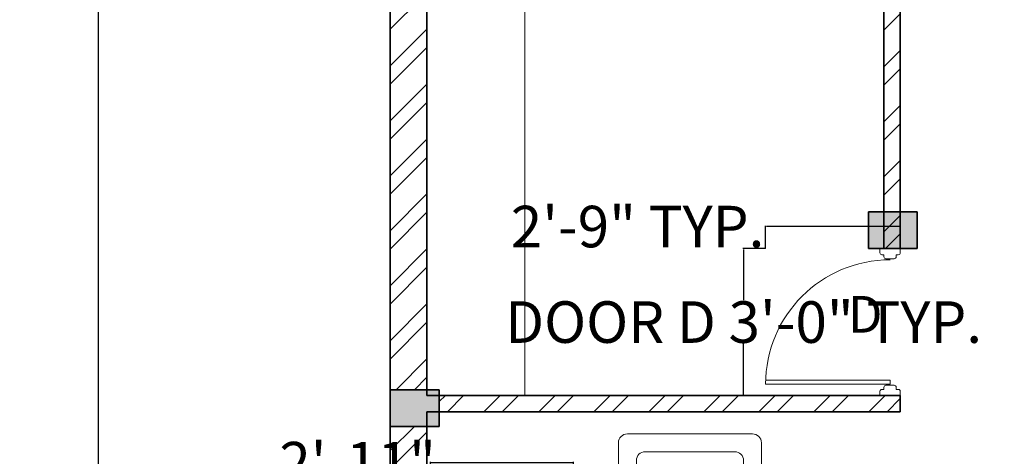
# Model space of a CAD drawing. Units: inches. Extents: x 2379 to 3013, y 1431 to 2110.
# Tile 3 of 10: x 2379 to 2620, y 1795 to 1902. Entities that reach past the tile are written whole.
import ezdxf

# ---------------------------------------------------------------- set-up
doc = ezdxf.new("R2010")
doc.units = ezdxf.units.IN
for name, color, linetype, lineweight in [('00 FURNITURE', 15, 'Continuous', 15), ('A-ANNO-DIMS', 2, 'Continuous', 18), ('A-ANNO-TEXT', 7, 'Continuous', 18), ('A-COLS', 7, 'Continuous', 35), ('A-COLS-PATT', 252, 'Continuous', 13), ('A-DOOR', 4, 'Continuous', 18), ('A-FLOR-CASE', 8, 'Continuous', 18), ('A-WALL-PATT', 8, 'Continuous', 13), ('WALL', 7, 'Continuous', 35)]:
    doc.layers.add(name, color=color, linetype=linetype, lineweight=lineweight)
doc.styles.get("Standard").update_dxf_attribs({"font": 'arial.ttf'})
doc.dimstyles.get("Standard").update_dxf_attribs({"dimtxt": 10.18, "dimasz": 0.18, "dimexe": 0.18, "dimexo": 0.0625, "dimgap": 0.09, "dimtad": 0, "dimtih": 1, "dimtoh": 1, "dimdec": 0, "dimzin": 0, "dimdsep": 46, "dimlunit": 3, "dimtxsty": 'Standard', "dimcen": 0.09, "dimadec": 0, "dimazin": 0, "dimtfac": 1, "dimtdec": 0, "dimtofl": 0, "dimtmove": 0, "dimatfit": 3, "dimfxl": 1, "dimtolj": 1, "dimtzin": 0, "dimarcsym": 0})

# ---------------------------------------------------------------- blocks, each defined once
blk = doc.blocks.new('column')
for p, q in [((2588.21, 2021.79), (2597.21, 2021.79)), ((2588.21, 2009.79), (2588.21, 2021.79)), ((2597.21, 2021.79), (2597.21, 2009.79)), ((2597.21, 2009.79), (2588.21, 2009.79))]:
    blk.add_line(p, q)
blk = doc.blocks.new('DDD')
at = {"layer": '00 FURNITURE'}
for p, q in [((-12579.77, -15859.53), (-12579.77, -15829.05)), ((-12578.77, -15859.53), (-12578.77, -15829.03)), ((-12612.02, -15857.03), (-12612.02, -15862.03)), ((-12611.02, -15857.03), (-12612.02, -15857.03)), ((-12577.02, -15857.03), (-12576.02, -15857.03)), ((-12576.02, -15857.03), (-12576.02, -15862.03)), ((-12610.52, -15858.03), (-12610.52, -15857.53)), ((-12578.77, -15859.53), (-12579.77, -15859.53)), ((-12577.52, -15858.03), (-12577.52, -15857.53)), ((-12612.02, -15862.03), (-12611.02, -15862.03)), ((-12610.52, -15861.53), (-12610.52, -15861.03)), ((-12577.52, -15861.53), (-12577.52, -15861.03)), ((-12576.02, -15862.03), (-12577.02, -15862.03))]:
    blk.add_line(p, q, dxfattribs=at)
for points in [[(-12610.52, -15861.03), (-12610.02, -15861.03, 0.414214), (-12609.52, -15860.53), (-12609.52, -15858.53, 0.414214), (-12610.02, -15858.03), (-12610.52, -15858.03)], [(-12577.52, -15861.03), (-12578.02, -15861.03, -0.414214), (-12578.52, -15860.53), (-12578.52, -15858.53, -0.414214), (-12578.02, -15858.03), (-12577.52, -15858.03)]]:
    blk.add_lwpolyline(points, format="xyb", dxfattribs=at)
for centre, radius, start, end in [((-12578.77, -15859.53), 30.5, 90, 180), ((-12611.02, -15857.53), 0.5, 0, 90), ((-12577.02, -15857.53), 0.5, 90, 180), ((-12611.02, -15861.53), 0.5, 270, 0), ((-12577.02, -15861.53), 0.5, 180, 270)]:
    blk.add_arc(centre, radius, start, end, dxfattribs=at)
blk = doc.blocks.new('*D13')
at = {"layer": 'A-ANNO-DIMS', "color": 0, "lineweight": -2, "transparency": 16777216}
for p, q in [((2469.57, 2021.61), (2397.82, 2021.61)), ((2398, 2021.43), (2398, 1755.4)), ((2398, 1478.79), (2398, 1744.82)), ((2469.57, 1478.61), (2397.82, 1478.61))]:
    blk.add_line(p, q, dxfattribs=at)
at = {"layer": 'A-ANNO-DIMS', "color": 0, "transparency": 16777216}
for points in [[(2397.97, 2021.43), (2398.03, 2021.43), (2398, 2021.61)], [(2397.97, 1478.79), (2398.03, 1478.79), (2398, 1478.61)]]:
    blk.add_solid(points, dxfattribs=at)
at = {"layer": 'Defpoints', "color": 0, "transparency": 16777216}
for p in [(2469.63, 2021.61), (2398, 1478.61), (2469.63, 1478.61)]:
    blk.add_point(p, dxfattribs=at)
at = {"layer": 'A-ANNO-DIMS', "color": 0, "transparency": 16777216, "insert": (2398, 1750.11), "char_height": 10.18, "attachment_point": 5}
blk.add_mtext('\\A1;45\'-3"', dxfattribs=at)
blk = doc.blocks.new('CHAIR-LOUNGE')
for p, q in [((32.85, 35.04), (2.19, 35.04)), ((0, 32.85), (0, 6.57)), ((35.04, 6.57), (35.04, 32.85)), ((28.47, 30.66), (6.57, 30.66)), ((4.38, 28.47), (4.38, 2.19)), ((30.66, 2.19), (30.66, 28.47)), ((30.66, 26.28), (4.38, 26.28)), ((2.19, 4.38), (4.38, 4.38)), ((30.66, 4.38), (32.85, 4.38)), ((6.57, 0), (28.47, 0))]:
    blk.add_line(p, q)
for centre, start, end in [((2.19, 32.85), 90, 180), ((32.85, 32.85), 0, 90), ((6.57, 28.47), 90, 180), ((28.47, 28.47), 0, 90), ((2.19, 6.57), 180, 270), ((32.85, 6.57), 270, 0), ((6.57, 2.19), 180, 270), ((28.47, 2.19), 270, 0)]:
    blk.add_arc(centre, 2.19, start, end)
blk = doc.blocks.new('*D24')
at = {"layer": 'A-ANNO-DIMS', "color": 0, "lineweight": -2, "transparency": 16777216}
for p, q in [((2561.57, 1845.61), (2556.05, 1845.61)), ((2556.23, 1845.43), (2556.23, 1832.97)), ((2556.23, 1809.79), (2556.23, 1822.25)), ((2561.57, 1809.61), (2556.05, 1809.61))]:
    blk.add_line(p, q, dxfattribs=at)
at = {"layer": 'A-ANNO-DIMS', "color": 0, "transparency": 16777216}
for points in [[(2556.2, 1845.43), (2556.26, 1845.43), (2556.23, 1845.61)], [(2556.2, 1809.79), (2556.26, 1809.79), (2556.23, 1809.61)]]:
    blk.add_solid(points, dxfattribs=at)
at = {"layer": 'Defpoints', "color": 0, "transparency": 16777216}
for p in [(2561.63, 1845.61), (2556.23, 1809.61), (2561.63, 1809.61)]:
    blk.add_point(p, dxfattribs=at)
at = {"layer": 'A-ANNO-DIMS', "color": 0, "transparency": 16777216, "insert": (2556.23, 1827.61), "char_height": 10.18, "attachment_point": 5}
blk.add_mtext('\\A1;DOOR D 3\'-0" TYP.', dxfattribs=at)
blk = doc.blocks.new('*D25')
at = {"layer": 'A-ANNO-DIMS', "color": 0, "lineweight": -2, "transparency": 16777216}
for p, q in [((2561.63, 1851.01), (2561.45, 1851.01)), ((2561.63, 1845.67), (2561.63, 1851.19)), ((2594.45, 1851.01), (2561.81, 1851.01)), ((2594.63, 1845.67), (2594.63, 1851.19))]:
    blk.add_line(p, q, dxfattribs=at)
at = {"layer": 'A-ANNO-DIMS', "color": 0, "transparency": 16777216}
for points in [[(2561.81, 1851.04), (2561.81, 1850.98), (2561.63, 1851.01)], [(2594.45, 1851.04), (2594.45, 1850.98), (2594.63, 1851.01)]]:
    blk.add_solid(points, dxfattribs=at)
at = {"layer": 'Defpoints', "color": 0, "transparency": 16777216}
for p in [(2561.63, 1851.01), (2561.63, 1845.61), (2594.63, 1845.61)]:
    blk.add_point(p, dxfattribs=at)
at = {"layer": 'A-ANNO-DIMS', "color": 0, "transparency": 16777216, "insert": (2530.25, 1851.01), "char_height": 10.18, "attachment_point": 5}
blk.add_mtext('\\A1;2\'-9" TYP.', dxfattribs=at)
blk = doc.blocks.new('*D37')
at = {"layer": 'A-ANNO-DIMS', "color": 0, "lineweight": -2, "transparency": 16777216}
for p, q in [((2479.47, 1793.16), (2479.29, 1793.16)), ((2479.47, 1780.23), (2479.47, 1793.34)), ((2514.33, 1793.16), (2479.65, 1793.16)), ((2514.51, 1780.23), (2514.51, 1793.34))]:
    blk.add_line(p, q, dxfattribs=at)
at = {"layer": 'A-ANNO-DIMS', "color": 0, "transparency": 16777216}
for points in [[(2479.65, 1793.19), (2479.65, 1793.13), (2479.47, 1793.16)], [(2514.33, 1793.19), (2514.33, 1793.13), (2514.51, 1793.16)]]:
    blk.add_solid(points, dxfattribs=at)
at = {"layer": 'Defpoints', "color": 0, "transparency": 16777216}
for p in [(2479.47, 1793.16), (2479.47, 1780.16), (2514.51, 1780.16)]:
    blk.add_point(p, dxfattribs=at)
at = {"layer": 'A-ANNO-DIMS', "color": 0, "transparency": 16777216, "insert": (2461.63, 1793.16), "char_height": 10.18, "attachment_point": 5}
blk.add_mtext('\\A1;2\'-11"', dxfattribs=at)

msp = doc.modelspace()

# ---------------------------------------------------------------- hatches: boundary and pattern name
at = {"layer": 'A-COLS-PATT'}
h = msp.add_hatch(color=256, dxfattribs=at)
h.dxf.hatch_style = 1
h.paths.add_polyline_path([(2937.62, 1660.61), (2925.62, 1660.61), (2925.62, 1651.61), (2937.62, 1651.61)])
h.paths.add_polyline_path([(2481.63, 1809.61), (2478.63, 1809.61), (2478.63, 1811.02), (2469.63, 1811.02), (2469.63, 1802.02), (2478.63, 1802.02), (2478.63, 1805.61), (2481.63, 1805.61)])
h.paths.add_polyline_path([(2481.63, 1811.02), (2478.63, 1811.02), (2478.63, 1809.61), (2481.63, 1809.61)], flags=17)
h.paths.add_polyline_path([(2481.63, 1805.61), (2478.63, 1805.61), (2478.63, 1802.02), (2481.63, 1802.02)], flags=17)
h.paths.add_polyline_path([(2481.63, 1660.61), (2469.63, 1660.61), (2469.63, 1651.61), (2481.63, 1651.61)])
h.paths.add_polyline_path([(2692.07, 1660.61), (2688.63, 1660.61), (2688.63, 1663.61), (2684.63, 1663.61), (2684.63, 1660.61), (2683.07, 1660.61), (2683.07, 1651.61), (2692.07, 1651.61)])
h.paths.add_polyline_path([(2692.07, 1663.61), (2688.63, 1663.61), (2688.63, 1660.61), (2692.07, 1660.61)], flags=17)
h.paths.add_polyline_path([(2684.63, 1663.61), (2683.07, 1663.61), (2683.07, 1660.61), (2684.63, 1660.61)], flags=17)
h.paths.add_polyline_path([(2770.63, 1660.61), (2767.63, 1660.61), (2767.63, 1663.61), (2763.63, 1663.61), (2763.63, 1660.61), (2761.63, 1660.61), (2761.63, 1651.61), (2763.63, 1651.61), (2767.63, 1651.61), (2767.63, 1651.61), (2770.63, 1651.61)])
h.paths.add_polyline_path([(2770.63, 1663.61), (2767.63, 1663.61), (2767.63, 1660.61), (2770.63, 1660.61)], flags=17)
h.paths.add_polyline_path([(2763.63, 1663.61), (2761.63, 1663.61), (2761.63, 1660.61), (2763.63, 1660.61)], flags=17)
h.paths.add_polyline_path([(2937.63, 1813.62), (2928.63, 1813.62), (2928.63, 1810.61), (2925.63, 1810.61), (2925.63, 1806.61), (2928.63, 1806.61), (2928.63, 1804.62), (2937.63, 1804.62)], flags=17)
h.paths.add_polyline_path([(2937.63, 1813.62), (2928.63, 1813.62), (2928.63, 1810.61), (2925.63, 1810.61), (2925.63, 1804.62), (2937.63, 1804.62)], flags=17)
h.paths.add_polyline_path([(2928.63, 1813.62), (2925.63, 1813.62), (2925.63, 1810.61), (2928.63, 1810.61)], flags=0)
h.paths.add_polyline_path([(2937.63, 1863.8), (2928.63, 1863.8), (2928.63, 1862.61), (2925.63, 1862.61), (2925.63, 1858.61), (2928.63, 1858.61), (2928.63, 1854.8), (2937.63, 1854.8)])
h.paths.add_polyline_path([(2928.63, 1863.8), (2925.63, 1863.8), (2925.63, 1862.61), (2928.63, 1862.61)], flags=17)
h.paths.add_polyline_path([(2928.63, 1858.61), (2925.63, 1858.61), (2925.63, 1854.8), (2928.63, 1854.8)], flags=17)
h.paths.add_polyline_path([(2937.63, 2021.61), (2928.63, 2021.61), (2928.63, 2012.61), (2928.63, 2012.61), (2928.63, 2009.61), (2937.63, 2009.61)])
h.paths.add_polyline_path([(2770.27, 2021.61), (2761.27, 2021.61), (2761.27, 2012.61), (2763.63, 2012.61), (2763.63, 2009.61), (2767.63, 2009.61), (2767.63, 2012.61), (2770.27, 2012.61)])
h.paths.add_polyline_path([(2763.63, 2012.61), (2761.27, 2012.61), (2761.27, 2009.61), (2763.63, 2009.61)], flags=17)
h.paths.add_polyline_path([(2770.27, 2012.61), (2767.63, 2012.61), (2767.63, 2009.61), (2770.27, 2009.61)], flags=17)
h.paths.add_polyline_path([(2597.21, 2021.61), (2588.21, 2021.61), (2588.21, 2012.61), (2590.63, 2012.61), (2590.63, 2009.61), (2594.63, 2009.61), (2594.63, 2012.61), (2597.21, 2012.61)])
h.paths.add_polyline_path([(2590.63, 2012.61), (2588.21, 2012.61), (2588.21, 2009.61), (2590.63, 2009.61)], flags=17)
h.paths.add_polyline_path([(2597.21, 2012.61), (2594.63, 2012.61), (2594.63, 2009.61), (2597.21, 2009.61)], flags=17)
h = msp.add_hatch(color=256, dxfattribs=at)
h.dxf.hatch_style = 1
h.paths.add_polyline_path([(2937.63, 1813.62), (2928.63, 1813.62), (2928.63, 1810.61), (2925.63, 1810.61), (2925.63, 1806.61), (2928.63, 1806.61), (2928.63, 1804.62), (2937.63, 1804.62)])
h.paths.add_polyline_path([(2928.63, 1813.62), (2925.63, 1813.62), (2925.63, 1810.61), (2928.63, 1810.61)], flags=17)
h.paths.add_polyline_path([(2693.63, 1810.71), (2684.63, 1810.71), (2684.63, 1810.61), (2688.63, 1810.61), (2688.63, 1798.71), (2693.63, 1798.71)])
h.paths.add_polyline_path([(2688.63, 1810.61), (2684.63, 1810.61), (2684.63, 1798.71), (2688.63, 1798.71)], flags=17)
h.paths.add_polyline_path([(2772.63, 1806.61), (2767.63, 1806.61), (2767.63, 1798.71), (2772.63, 1798.71)], flags=17)
h.paths.add_polyline_path([(2772.63, 1810.61), (2763.63, 1810.61), (2763.63, 1798.71), (2767.63, 1798.71), (2767.63, 1806.61), (2772.63, 1806.61)])
h.paths.add_polyline_path([(2773.54, 1858.61), (2763.63, 1858.61), (2763.63, 1862.61), (2761.54, 1862.61), (2761.54, 1853.61), (2773.54, 1853.61)])
h.paths.add_polyline_path([(2773.54, 1862.61), (2763.63, 1862.61), (2763.63, 1858.61), (2773.54, 1858.61)], flags=17)
h.paths.add_polyline_path([(2598.8, 1854.61), (2594.63, 1854.61), (2594.63, 1845.61), (2598.8, 1845.61)])
h.paths.add_polyline_path([(2594.63, 1854.61), (2590.63, 1854.61), (2590.63, 1845.61), (2594.63, 1845.61)])
h.paths.add_polyline_path([(2590.63, 1854.61), (2586.8, 1854.61), (2586.8, 1845.61), (2590.63, 1845.61)])
at = {"layer": 'A-WALL-PATT'}
h = msp.add_hatch(dxfattribs=at)
h.set_pattern_fill('ANSI32', color=256)
h.paths.add_polyline_path([(2925.63, 1862.61), (2815.63, 1862.61), (2815.63, 1858.61), (2827.63, 1858.61), (2827.63, 1810.61), (2815.63, 1810.61), (2815.63, 1806.61), (2850.78, 1806.61), (2850.78, 1810.61), (2831.63, 1810.61), (2831.63, 1858.61), (2925.63, 1858.61)])
h.paths.add_polyline_path([(2925.63, 1810.61), (2880.78, 1810.61), (2880.78, 1806.61), (2925.63, 1806.61)], flags=17)
h.paths.add_polyline_path([(2633.75, 1660.61), (2594.63, 1660.61), (2481.63, 1660.61), (2481.63, 1651.61), (2588.63, 1651.61), (2588.63, 1570.61), (2624.28, 1570.61), (2624.28, 1574.61), (2592.63, 1574.61), (2592.63, 1651.61), (2633.75, 1651.61)])
h.paths.add_polyline_path([(2594.63, 1809.61), (2481.63, 1809.61), (2481.63, 1805.61), (2594.63, 1805.61)])
h.paths.add_polyline_path([(2594.63, 2012.61), (2597.21, 2012.61), (2597.21, 2021.61), (2588.21, 2021.61), (2588.21, 2012.61), (2590.63, 2012.61), (2590.63, 1845.61), (2594.63, 1845.61)])
h.paths.add_polyline_path([(2767.63, 2012.61), (2770.27, 2012.61), (2770.27, 2021.61), (2761.27, 2021.61), (2761.27, 2012.61), (2763.63, 2012.61), (2763.63, 1928.61), (2691.63, 1928.61), (2643.63, 1928.61), (2643.63, 1924.61), (2691.63, 1924.61), (2763.63, 1924.61), (2763.63, 1858.61), (2779.63, 1858.61), (2779.63, 1862.61), (2767.63, 1862.61)])
h.paths.add_polyline_path([(2613.63, 2012.61), (2613.63, 2021.61), (2597.21, 2021.61), (2597.21, 2012.61)])
h.paths.add_polyline_path([(2508.33, 2012.61), (2508.33, 2021.61), (2478.63, 2021.61), (2478.63, 2012.61)])
h.paths.add_polyline_path([(2556.33, 2021.61), (2556.33, 2012.61), (2588.21, 2012.61), (2588.21, 2021.61)])
h.paths.add_polyline_path([(2659.15, 2012.61), (2659.15, 2021.61), (2643.63, 2021.61), (2643.63, 1958.61), (2661.63, 1958.61), (2661.63, 1962.61), (2647.63, 1962.61), (2647.63, 2012.61)])
h.paths.add_polyline_path([(2714.17, 2012.61), (2714.17, 2021.61), (2683.15, 2021.61), (2683.15, 2012.61), (2691.63, 2012.61), (2691.63, 1958.61), (2695.63, 1958.61), (2695.63, 2012.61)])
h.paths.add_polyline_path([(2738.17, 2021.61), (2738.17, 2012.61), (2761.27, 2012.61), (2761.27, 2021.61)])
h.paths.add_polyline_path([(2820.76, 2012.61), (2820.76, 2021.61), (2770.27, 2021.61), (2770.27, 2012.61)])
h.paths.add_polyline_path([(2868.76, 2021.61), (2868.76, 2012.61), (2928.63, 2012.61), (2928.63, 2021.61)])
h.paths.add_polyline_path([(2928.63, 1962.9), (2937.63, 1962.9), (2937.63, 2009.61), (2928.63, 2009.61)])
h.paths.add_polyline_path([(2937.63, 1914.9), (2928.63, 1914.9), (2928.63, 1863.8), (2937.63, 1863.8)])
h.paths.add_polyline_path([(2928.63, 1846.59), (2937.63, 1846.59), (2937.63, 1854.8), (2928.63, 1854.8)])
h.paths.add_polyline_path([(2937.63, 1822.59), (2928.63, 1822.59), (2928.63, 1813.62), (2937.63, 1813.62)])
h.paths.add_polyline_path([(2928.63, 1778.48), (2937.63, 1778.48), (2937.63, 1813.62), (2928.63, 1813.62), (2928.63, 1810.61), (2925.63, 1810.61), (2925.63, 1806.61), (2928.63, 1806.61)])
h.paths.add_polyline_path([(2816.22, 1651.61), (2816.22, 1660.61), (2767.63, 1660.61), (2767.63, 1806.61), (2779.63, 1806.61), (2779.63, 1810.61), (2763.63, 1810.61), (2763.63, 1660.61), (2688.63, 1660.61), (2688.63, 1810.61), (2684.63, 1810.61), (2684.63, 1660.61), (2669.75, 1660.61), (2669.75, 1651.61), (2763.63, 1651.61), (2763.63, 1574.61), (2672.28, 1574.61), (2672.28, 1570.61), (2767.63, 1570.61), (2767.63, 1651.61)])
h.paths.add_polyline_path([(2864.22, 1660.61), (2864.22, 1651.61), (2937.63, 1651.61), (2937.63, 1730.48), (2928.63, 1730.48), (2928.63, 1660.61)])
h.paths.add_polyline_path([(2469.63, 1975.19), (2478.63, 1975.19), (2478.63, 2009.61), (2469.63, 2009.61)])
h.paths.add_polyline_path([(2478.63, 1927.19), (2469.63, 1927.19), (2469.63, 1811.02), (2478.63, 1811.02)])
h.paths.add_polyline_path([(2469.63, 1758.04), (2478.63, 1758.04), (2478.63, 1802.02), (2469.63, 1802.02)])
h.paths.add_polyline_path([(2478.63, 1710.04), (2469.63, 1710.04), (2469.63, 1660.61), (2478.63, 1660.61)])

# ---------------------------------------------------------------- linework, layer by layer
at = {"layer": 'A-FLOR-CASE'}
msp.add_line((2502.63, 1809.61), (2502.63, 1988.61), dxfattribs=at)
at = {"layer": 'WALL'}
for p, q in [((2590.63, 1845.61), (2590.63, 2012.61)), ((2594.63, 1845.61), (2594.63, 2012.61)), ((2469.63, 1758.04), (2469.63, 1927.19)), ((2478.63, 1809.61), (2478.63, 1927.19)), ((2590.63, 1845.61), (2594.63, 1845.61)), ((2478.63, 1809.61), (2594.63, 1809.61)), ((2594.63, 1805.61), (2594.63, 1809.61)), ((2478.63, 1805.61), (2594.63, 1805.61)), ((2478.63, 1758.04), (2478.63, 1805.61))]:
    msp.add_line(p, q, dxfattribs=at)

# ---------------------------------------------------------------- block references
at = {"layer": '00 FURNITURE'}
msp.add_blockref('CHAIR-LOUNGE', (2525.56, 1765.19), dxfattribs=at)
at = {"layer": 'A-COLS', "rotation": 270}
for p in [(577.02, 4442.82), (459.84, 4399.23)]:
    msp.add_blockref('column', p, dxfattribs=at)
at = {"layer": 'A-DOOR', "xscale": -1, "rotation": 90}
msp.add_blockref('DDD', (-13267.4, -10766.41), dxfattribs=at)

# ---------------------------------------------------------------- texts
at = {"layer": 'A-ANNO-TEXT', "insert": (2581.83, 1834.01), "char_height": 9, "attachment_point": 1}
msp.add_mtext_dynamic_manual_height_columns('D', width=106.8919, gutter_width=12.5, heights=[0], dxfattribs=at)

# ---------------------------------------------------------------- dimensions: what is measured, and where the dimension line sits
at = {"layer": 'A-ANNO-DIMS'}
for base, p1, p2, angle, override, picture, middle in [((2398, 1478.61), (2469.63, 2021.61), (2469.63, 1478.61), 90, {"dimclrd": 0, "dimclre": 0, "dimclrt": 0}, '*D13', (2398, 1750.11)), ((2479.47, 1793.16), (2514.51, 1780.16), (2479.47, 1780.16), 180, {"dimdec": 1, "dimlfac": 1, "dimrnd": 0, "dimzin": 1, "dimdsep": 46, "dimlunit": 4, "dimfrac": 2}, '*D37', (2461.63, 1793.16))]:
    dim = msp.add_linear_dim(base=base, p1=p1, p2=p2, angle=angle, dimstyle='Standard', override=override, dxfattribs=at)
    dim.commit()
    dim.dimension.update_dxf_attribs({"geometry": picture, "text_midpoint": middle})
for base, p1, p2, angle, text, picture, middle in [((2561.63, 1851.01), (2594.63, 1845.61), (2561.63, 1845.61), 180, '<> TYP.', '*D25', (2530.25, 1851.01)), ((2556.23, 1809.61), (2561.63, 1845.61), (2561.63, 1809.61), 270, 'DOOR D <> TYP.', '*D24', (2556.23, 1827.61))]:
    dim = msp.add_linear_dim(base=base, p1=p1, p2=p2, angle=angle, text=text, dimstyle='Standard', override={"dimdec": 1, "dimlfac": 1, "dimrnd": 0, "dimzin": 1, "dimdsep": 46, "dimlunit": 4, "dimfrac": 2}, dxfattribs=at)
    dim.commit()
    dim.dimension.update_dxf_attribs({"geometry": picture, "text_midpoint": middle})

doc.saveas('drawing.dxf')
